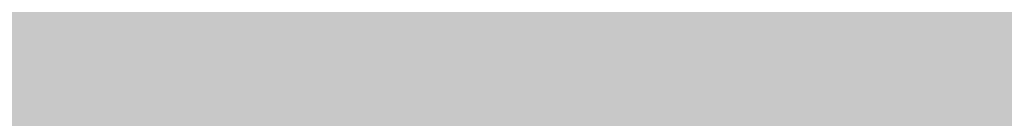
# Model space of a CAD drawing. Units: millimetres. Extents: x -22994 to 29398, y -19990 to 20176.
# Tile 87 of 135: x 229.428 to 230.597, y 83.328 to 83.446. Entities that reach past the tile are written whole.
import ezdxf
from ezdxf import colors
from ezdxf.entities.mleader import LeaderData, LeaderLine
from ezdxf.math import Vec2, Vec3

# ---------------------------------------------------------------- set-up
doc = ezdxf.new("R2010")
doc.units = ezdxf.units.MM
doc.header["$MEASUREMENT"] = 0
doc.layers.add('M-ANNO-TEXT', color=7, linetype='Continuous', lineweight=25)
doc.layers.add('M-DIMS', color=2, linetype='Continuous', lineweight=18)
doc.styles.get("Standard").update_dxf_attribs({"font": 'arial.ttf'})
doc.dimstyles.get("Standard").update_dxf_attribs({"dimtxt": 0.18, "dimasz": 10000, "dimexe": 0.18, "dimexo": 0.0625, "dimgap": 0.09, "dimtad": 0, "dimtih": 1, "dimtoh": 1, "dimdec": 0, "dimzin": 0, "dimdsep": 46, "dimtxsty": 'Standard', "dimcen": 0.09, "dimadec": 0, "dimazin": 0, "dimtfac": 1, "dimtdec": 0, "dimtofl": 0, "dimtmove": 0, "dimatfit": 3, "dimfxl": 1, "dimtolj": 1, "dimtzin": 0, "dimlwd": 30, "dimarcsym": 0})

# ---------------------------------------------------------------- blocks, each defined once
blk = doc.blocks.new('*D2')
at = {"layer": 'Defpoints', "color": 0, "transparency": 16777216}
for p in [(6.6773, 10.2713), (290.852, 10.2713), (290.852, -5.0787)]:
    blk.add_point(p, dxfattribs=at)
at = {"layer": 'M-DIMS', "color": 0, "lineweight": -2, "transparency": 16777216}
for p, q in [((6.6773, 10.2088), (6.6773, -5.2587)), ((290.852, 10.2088), (290.852, -5.2587))]:
    blk.add_line(p, q, dxfattribs=at)
at = {"layer": 'M-DIMS', "color": 0, "lineweight": 30, "transparency": 16777216}
for p, q in [((-9993.3227, -5.0787), (-19993.3227, -5.0787)), ((10290.852, -5.0787), (20290.852, -5.0787))]:
    blk.add_line(p, q, dxfattribs=at)
at = {"layer": 'M-DIMS', "color": 0, "transparency": 16777216}
for points in [[(-9993.3227, 1661.5879), (-9993.3227, -1671.7454), (6.6773, -5.0787)], [(10290.852, 1661.5879), (10290.852, -1671.7454), (290.852, -5.0787)]]:
    blk.add_solid(points, dxfattribs=at)
at = {"layer": 'M-DIMS', "color": 0, "transparency": 16777216, "insert": (148.7647, -5.0787), "char_height": 0.18, "attachment_point": 5}
blk.add_mtext('\\A1;284.2', dxfattribs=at)
blk = doc.blocks.new('*D3')
at = {"layer": 'Defpoints', "color": 0, "transparency": 16777216}
for p in [(110.2647, 204.1654), (110.2647, 176.3662), (95.8327, 127.967)]:
    blk.add_point(p, dxfattribs=at)
at = {"layer": 'M-DIMS', "color": 0, "lineweight": -2, "transparency": 16777216}
for p, q in [((95.8327, 128.0295), (95.8327, 204.3454)), ((110.2647, 176.4287), (110.2647, 204.3454))]:
    blk.add_line(p, q, dxfattribs=at)
at = {"layer": 'M-DIMS', "color": 0, "lineweight": 30, "transparency": 16777216}
for p, q in [((-9904.1673, 204.1654), (-19904.1673, 204.1654)), ((10110.2647, 204.1654), (20110.2647, 204.1654))]:
    blk.add_line(p, q, dxfattribs=at)
at = {"layer": 'M-DIMS', "color": 0, "transparency": 16777216}
for points in [[(-9904.1673, 1870.8321), (-9904.1673, -1462.5013), (95.8327, 204.1654)], [(10110.2647, 1870.8321), (10110.2647, -1462.5013), (110.2647, 204.1654)]]:
    blk.add_solid(points, dxfattribs=at)
at = {"layer": 'M-DIMS', "color": 0, "transparency": 16777216, "insert": (103.0487, 204.1654), "char_height": 0.18, "attachment_point": 5}
blk.add_mtext('\\A1;14.432', dxfattribs=at)
blk = doc.blocks.new('*D4')
at = {"layer": 'Defpoints', "color": 0, "transparency": 16777216}
for p in [(116.2647, 204.1654), (110.2647, 176.3662), (116.2647, 176.3662)]:
    blk.add_point(p, dxfattribs=at)
at = {"layer": 'M-DIMS', "color": 0, "lineweight": -2, "transparency": 16777216}
for p, q in [((110.2647, 176.4287), (110.2647, 204.3454)), ((116.2647, 176.4287), (116.2647, 204.3454))]:
    blk.add_line(p, q, dxfattribs=at)
at = {"layer": 'M-DIMS', "color": 0, "lineweight": 30, "transparency": 16777216}
for p, q in [((-9889.7353, 204.1654), (-19889.7353, 204.1654)), ((10116.2647, 204.1654), (20116.2647, 204.1654))]:
    blk.add_line(p, q, dxfattribs=at)
at = {"layer": 'M-DIMS', "color": 0, "transparency": 16777216}
for points in [[(-9889.7353, 1870.8321), (-9889.7353, -1462.5013), (110.2647, 204.1654)], [(10116.2647, 1870.8321), (10116.2647, -1462.5013), (116.2647, 204.1654)]]:
    blk.add_solid(points, dxfattribs=at)
at = {"layer": 'M-DIMS', "color": 0, "transparency": 16777216, "insert": (113.2647, 204.1654), "char_height": 0.18, "attachment_point": 5}
blk.add_mtext('\\A1;6', dxfattribs=at)
blk = doc.blocks.new('*D5')
at = {"layer": 'Defpoints', "color": 0, "transparency": 16777216}
for p in [(181.2647, 204.1654), (116.2647, 176.3662), (181.2647, 176.3662)]:
    blk.add_point(p, dxfattribs=at)
at = {"layer": 'M-DIMS', "color": 0, "lineweight": -2, "transparency": 16777216}
for p, q in [((116.2647, 176.4287), (116.2647, 204.3454)), ((181.2647, 176.4287), (181.2647, 204.3454))]:
    blk.add_line(p, q, dxfattribs=at)
at = {"layer": 'M-DIMS', "color": 0, "lineweight": 30, "transparency": 16777216}
for p, q in [((-9883.7353, 204.1654), (-19883.7353, 204.1654)), ((10181.2647, 204.1654), (20181.2647, 204.1654))]:
    blk.add_line(p, q, dxfattribs=at)
at = {"layer": 'M-DIMS', "color": 0, "transparency": 16777216}
for points in [[(-9883.7353, 1870.8321), (-9883.7353, -1462.5013), (116.2647, 204.1654)], [(10181.2647, 1870.8321), (10181.2647, -1462.5013), (181.2647, 204.1654)]]:
    blk.add_solid(points, dxfattribs=at)
at = {"layer": 'M-DIMS', "color": 0, "transparency": 16777216, "insert": (148.7647, 204.1654), "char_height": 0.18, "attachment_point": 5}
blk.add_mtext('\\A1;65', dxfattribs=at)
blk = doc.blocks.new('*D6')
at = {"layer": 'Defpoints', "color": 0, "transparency": 16777216}
for p in [(187.2647, 204.1654), (181.2647, 176.3662), (187.2647, 176.3662)]:
    blk.add_point(p, dxfattribs=at)
at = {"layer": 'M-DIMS', "color": 0, "lineweight": -2, "transparency": 16777216}
for p, q in [((181.2647, 176.4287), (181.2647, 204.3454)), ((187.2647, 176.4287), (187.2647, 204.3454))]:
    blk.add_line(p, q, dxfattribs=at)
at = {"layer": 'M-DIMS', "color": 0, "lineweight": 30, "transparency": 16777216}
for p, q in [((-9818.7353, 204.1654), (-19818.7353, 204.1654)), ((10187.2647, 204.1654), (20187.2647, 204.1654))]:
    blk.add_line(p, q, dxfattribs=at)
at = {"layer": 'M-DIMS', "color": 0, "transparency": 16777216}
for points in [[(-9818.7353, 1870.8321), (-9818.7353, -1462.5013), (181.2647, 204.1654)], [(10187.2647, 1870.8321), (10187.2647, -1462.5013), (187.2647, 204.1654)]]:
    blk.add_solid(points, dxfattribs=at)
at = {"layer": 'M-DIMS', "color": 0, "transparency": 16777216, "insert": (184.2647, 204.1654), "char_height": 0.18, "attachment_point": 5}
blk.add_mtext('\\A1;6', dxfattribs=at)
blk = doc.blocks.new('*D7')
at = {"layer": 'Defpoints', "color": 0, "transparency": 16777216}
for p in [(201.6967, 204.1654), (187.2647, 176.3662), (201.6967, 127.967)]:
    blk.add_point(p, dxfattribs=at)
at = {"layer": 'M-DIMS', "color": 0, "lineweight": -2, "transparency": 16777216}
for p, q in [((187.2647, 176.4287), (187.2647, 204.3454)), ((201.6967, 128.0295), (201.6967, 204.3454))]:
    blk.add_line(p, q, dxfattribs=at)
at = {"layer": 'M-DIMS', "color": 0, "lineweight": 30, "transparency": 16777216}
for p, q in [((-9812.7353, 204.1654), (-19812.7353, 204.1654)), ((10201.6967, 204.1654), (20201.6967, 204.1654))]:
    blk.add_line(p, q, dxfattribs=at)
at = {"layer": 'M-DIMS', "color": 0, "transparency": 16777216}
for points in [[(-9812.7353, 1870.8321), (-9812.7353, -1462.5013), (187.2647, 204.1654)], [(10201.6967, 1870.8321), (10201.6967, -1462.5013), (201.6967, 204.1654)]]:
    blk.add_solid(points, dxfattribs=at)
at = {"layer": 'M-DIMS', "color": 0, "transparency": 16777216, "insert": (194.4807, 204.1654), "char_height": 0.18, "attachment_point": 5}
blk.add_mtext('\\A1;14.432', dxfattribs=at)
blk = doc.blocks.new('*D8')
at = {"layer": 'Defpoints', "color": 0, "transparency": 16777216}
for p in [(227.6485, 204.1654), (227.6485, 146.7296), (201.6967, 127.967)]:
    blk.add_point(p, dxfattribs=at)
at = {"layer": 'M-DIMS', "color": 0, "lineweight": -2, "transparency": 16777216}
for p, q in [((201.6967, 128.0295), (201.6967, 204.3454)), ((227.6485, 146.7921), (227.6485, 204.3454))]:
    blk.add_line(p, q, dxfattribs=at)
at = {"layer": 'M-DIMS', "color": 0, "lineweight": 30, "transparency": 16777216}
for p, q in [((-9798.3033, 204.1654), (-19798.3033, 204.1654)), ((10227.6485, 204.1654), (20227.6485, 204.1654))]:
    blk.add_line(p, q, dxfattribs=at)
at = {"layer": 'M-DIMS', "color": 0, "transparency": 16777216}
for points in [[(-9798.3033, 1870.8321), (-9798.3033, -1462.5013), (201.6967, 204.1654)], [(10227.6485, 1870.8321), (10227.6485, -1462.5013), (227.6485, 204.1654)]]:
    blk.add_solid(points, dxfattribs=at)
at = {"layer": 'M-DIMS', "color": 0, "transparency": 16777216, "insert": (214.6726, 204.1654), "char_height": 0.18, "attachment_point": 5}
blk.add_mtext('\\A1;25.95', dxfattribs=at)
blk = doc.blocks.new('*D9')
at = {"layer": 'Defpoints', "color": 0, "transparency": 16777216}
for p in [(187.2647, 176.3662), (306.202, 176.3662), (290.852, 10.2713)]:
    blk.add_point(p, dxfattribs=at)
at = {"layer": 'M-DIMS', "color": 0, "lineweight": 30, "transparency": 16777216}
for p, q in [((306.202, 10176.3662), (306.202, 20176.3662)), ((306.202, -9989.7287), (306.202, -19989.7287))]:
    blk.add_line(p, q, dxfattribs=at)
at = {"layer": 'M-DIMS', "color": 0, "lineweight": -2, "transparency": 16777216}
for p, q in [((187.3272, 176.3662), (306.382, 176.3662)), ((290.9145, 10.2713), (306.382, 10.2713))]:
    blk.add_line(p, q, dxfattribs=at)
at = {"layer": 'M-DIMS', "color": 0, "transparency": 16777216}
for points in [[(-1360.4646, 10176.3662), (1972.8687, 10176.3662), (306.202, 176.3662)], [(-1360.4646, -9989.7287), (1972.8687, -9989.7287), (306.202, 10.2713)]]:
    blk.add_solid(points, dxfattribs=at)
at = {"layer": 'M-DIMS', "color": 0, "transparency": 16777216, "insert": (306.202, 93.3187), "char_height": 0.18, "attachment_point": 5}
blk.add_mtext('\\A1;166.1', dxfattribs=at)
blk = doc.blocks.new('*D10')
at = {"layer": 'Defpoints', "color": 0, "transparency": 16777216}
for p in [(125.6498, 136.0713), (133.3459, 136.0713), (133.3459, -5.0787)]:
    blk.add_point(p, dxfattribs=at)
at = {"layer": 'M-DIMS', "color": 0, "lineweight": -2, "transparency": 16777216}
for p, q in [((125.6498, 136.0088), (125.6498, -5.2587)), ((133.3459, 136.0088), (133.3459, -5.2587))]:
    blk.add_line(p, q, dxfattribs=at)
at = {"layer": 'M-DIMS', "color": 0, "lineweight": 30, "transparency": 16777216}
for p, q in [((-9874.3502, -5.0787), (-19874.3502, -5.0787)), ((10133.3459, -5.0787), (20133.3459, -5.0787))]:
    blk.add_line(p, q, dxfattribs=at)
at = {"layer": 'M-DIMS', "color": 0, "transparency": 16777216}
for points in [[(-9874.3502, 1661.5879), (-9874.3502, -1671.7454), (125.6498, -5.0787)], [(10133.3459, 1661.5879), (10133.3459, -1671.7454), (133.3459, -5.0787)]]:
    blk.add_solid(points, dxfattribs=at)
at = {"layer": 'M-DIMS', "color": 0, "transparency": 16777216, "insert": (129.4978, -5.0787), "char_height": 0.18, "attachment_point": 5}
blk.add_mtext('\\A1;7.696', dxfattribs=at)
blk = doc.blocks.new('*D11')
at = {"layer": 'Defpoints', "color": 0, "transparency": 16777216}
for p in [(133.3459, 136.0713), (135.6498, 136.0713), (135.6498, -5.0787)]:
    blk.add_point(p, dxfattribs=at)
at = {"layer": 'M-DIMS', "color": 0, "lineweight": -2, "transparency": 16777216}
for p, q in [((133.3459, 136.0088), (133.3459, -5.2587)), ((135.6498, 136.0088), (135.6498, -5.2587))]:
    blk.add_line(p, q, dxfattribs=at)
at = {"layer": 'M-DIMS', "color": 0, "lineweight": 30, "transparency": 16777216}
for p, q in [((-9866.6541, -5.0787), (-19866.6541, -5.0787)), ((10135.6498, -5.0787), (20135.6498, -5.0787))]:
    blk.add_line(p, q, dxfattribs=at)
at = {"layer": 'M-DIMS', "color": 0, "transparency": 16777216}
for points in [[(-9866.6541, 1661.5879), (-9866.6541, -1671.7454), (133.3459, -5.0787)], [(10135.6498, 1661.5879), (10135.6498, -1671.7454), (135.6498, -5.0787)]]:
    blk.add_solid(points, dxfattribs=at)
at = {"layer": 'M-DIMS', "color": 0, "transparency": 16777216, "insert": (134.4978, -5.0787), "char_height": 0.18, "attachment_point": 5}
blk.add_mtext('\\A1;2.304', dxfattribs=at)
blk = doc.blocks.new('*D12')
at = {"layer": 'Defpoints', "color": 0, "transparency": 16777216}
for p in [(135.6498, 136.0713), (145.6498, 136.0713), (145.6498, -5.0787)]:
    blk.add_point(p, dxfattribs=at)
at = {"layer": 'M-DIMS', "color": 0, "lineweight": -2, "transparency": 16777216}
for p, q in [((135.6498, 136.0088), (135.6498, -5.2587)), ((145.6498, 136.0088), (145.6498, -5.2587))]:
    blk.add_line(p, q, dxfattribs=at)
at = {"layer": 'M-DIMS', "color": 0, "lineweight": 30, "transparency": 16777216}
for p, q in [((-9864.3502, -5.0787), (-19864.3502, -5.0787)), ((10145.6498, -5.0787), (20145.6498, -5.0787))]:
    blk.add_line(p, q, dxfattribs=at)
at = {"layer": 'M-DIMS', "color": 0, "transparency": 16777216}
for points in [[(-9864.3502, 1661.5879), (-9864.3502, -1671.7454), (135.6498, -5.0787)], [(10145.6498, 1661.5879), (10145.6498, -1671.7454), (145.6498, -5.0787)]]:
    blk.add_solid(points, dxfattribs=at)
at = {"layer": 'M-DIMS', "color": 0, "transparency": 16777216, "insert": (140.6498, -5.0787), "char_height": 0.18, "attachment_point": 5}
blk.add_mtext('\\A1;10', dxfattribs=at)
blk = doc.blocks.new('*D13')
at = {"layer": 'Defpoints', "color": 0, "transparency": 16777216}
for p in [(145.6498, 136.0713), (155.6498, 136.0713), (155.6498, -5.0787)]:
    blk.add_point(p, dxfattribs=at)
at = {"layer": 'M-DIMS', "color": 0, "lineweight": -2, "transparency": 16777216}
for p, q in [((145.6498, 136.0088), (145.6498, -5.2587)), ((155.6498, 136.0088), (155.6498, -5.2587))]:
    blk.add_line(p, q, dxfattribs=at)
at = {"layer": 'M-DIMS', "color": 0, "lineweight": 30, "transparency": 16777216}
for p, q in [((-9854.3502, -5.0787), (-19854.3502, -5.0787)), ((10155.6498, -5.0787), (20155.6498, -5.0787))]:
    blk.add_line(p, q, dxfattribs=at)
at = {"layer": 'M-DIMS', "color": 0, "transparency": 16777216}
for points in [[(-9854.3502, 1661.5879), (-9854.3502, -1671.7454), (145.6498, -5.0787)], [(10155.6498, 1661.5879), (10155.6498, -1671.7454), (155.6498, -5.0787)]]:
    blk.add_solid(points, dxfattribs=at)
at = {"layer": 'M-DIMS', "color": 0, "transparency": 16777216, "insert": (150.6498, -5.0787), "char_height": 0.18, "attachment_point": 5}
blk.add_mtext('\\A1;10', dxfattribs=at)
blk = doc.blocks.new('*D14')
at = {"layer": 'Defpoints', "color": 0, "transparency": 16777216}
for p in [(155.6498, 136.0713), (165.6498, 136.0713), (165.6498, -5.0787)]:
    blk.add_point(p, dxfattribs=at)
at = {"layer": 'M-DIMS', "color": 0, "lineweight": -2, "transparency": 16777216}
for p, q in [((155.6498, 136.0088), (155.6498, -5.2587)), ((165.6498, 136.0088), (165.6498, -5.2587))]:
    blk.add_line(p, q, dxfattribs=at)
at = {"layer": 'M-DIMS', "color": 0, "lineweight": 30, "transparency": 16777216}
for p, q in [((-9844.3502, -5.0787), (-19844.3502, -5.0787)), ((10165.6498, -5.0787), (20165.6498, -5.0787))]:
    blk.add_line(p, q, dxfattribs=at)
at = {"layer": 'M-DIMS', "color": 0, "transparency": 16777216}
for points in [[(-9844.3502, 1661.5879), (-9844.3502, -1671.7454), (155.6498, -5.0787)], [(10165.6498, 1661.5879), (10165.6498, -1671.7454), (165.6498, -5.0787)]]:
    blk.add_solid(points, dxfattribs=at)
at = {"layer": 'M-DIMS', "color": 0, "transparency": 16777216, "insert": (160.6498, -5.0787), "char_height": 0.18, "attachment_point": 5}
blk.add_mtext('\\A1;10', dxfattribs=at)
blk = doc.blocks.new('*D15')
at = {"layer": 'Defpoints', "color": 0, "transparency": 16777216}
for p in [(173.3459, 154.788), (173.3459, 136.0713), (306.202, 136.0713)]:
    blk.add_point(p, dxfattribs=at)
at = {"layer": 'M-DIMS', "color": 0, "lineweight": 30, "transparency": 16777216}
for p, q in [((306.202, 10154.788), (306.202, 20154.788)), ((306.202, -9863.9287), (306.202, -19863.9287))]:
    blk.add_line(p, q, dxfattribs=at)
at = {"layer": 'M-DIMS', "color": 0, "lineweight": -2, "transparency": 16777216}
for p, q in [((173.4084, 154.788), (306.382, 154.788)), ((173.4084, 136.0713), (306.382, 136.0713))]:
    blk.add_line(p, q, dxfattribs=at)
at = {"layer": 'M-DIMS', "color": 0, "transparency": 16777216}
for points in [[(-1360.4646, 10154.788), (1972.8687, 10154.788), (306.202, 154.788)], [(-1360.4646, -9863.9287), (1972.8687, -9863.9287), (306.202, 136.0713)]]:
    blk.add_solid(points, dxfattribs=at)
at = {"layer": 'M-DIMS', "color": 0, "transparency": 16777216, "insert": (306.202, 145.4297), "char_height": 0.18, "attachment_point": 5}
blk.add_mtext('\\A1;18.717', dxfattribs=at)
blk = doc.blocks.new('*D16')
at = {"layer": 'Defpoints', "color": 0, "transparency": 16777216}
for p in [(120.1702, 204.1654), (110.4658, 48.0349), (120.1702, 48.0349)]:
    blk.add_point(p, dxfattribs=at)
at = {"layer": 'M-DIMS', "color": 0, "lineweight": -2, "transparency": 16777216}
for p, q in [((110.4658, 48.0974), (110.4658, 204.3454)), ((120.1702, 48.0974), (120.1702, 204.3454))]:
    blk.add_line(p, q, dxfattribs=at)
at = {"layer": 'M-DIMS', "color": 0, "lineweight": 30, "transparency": 16777216}
for p, q in [((-9889.5342, 204.1654), (-19889.5342, 204.1654)), ((10120.1702, 204.1654), (20120.1702, 204.1654))]:
    blk.add_line(p, q, dxfattribs=at)
at = {"layer": 'M-DIMS', "color": 0, "transparency": 16777216}
for points in [[(-9889.5342, 1870.8321), (-9889.5342, -1462.5013), (110.4658, 204.1654)], [(10120.1702, 1870.8321), (10120.1702, -1462.5013), (120.1702, 204.1654)]]:
    blk.add_solid(points, dxfattribs=at)
at = {"layer": 'M-DIMS', "color": 0, "transparency": 16777216, "insert": (115.318, 204.1654), "char_height": 0.18, "attachment_point": 5}
blk.add_mtext('\\A1;9.704', dxfattribs=at)
blk = doc.blocks.new('*D17')
at = {"layer": 'Defpoints', "color": 0, "transparency": 16777216}
for p in [(126.1702, 204.1654), (120.1702, 48.0349), (126.1702, 48.0349)]:
    blk.add_point(p, dxfattribs=at)
at = {"layer": 'M-DIMS', "color": 0, "lineweight": -2, "transparency": 16777216}
for p, q in [((120.1702, 48.0974), (120.1702, 204.3454)), ((126.1702, 48.0974), (126.1702, 204.3454))]:
    blk.add_line(p, q, dxfattribs=at)
at = {"layer": 'M-DIMS', "color": 0, "lineweight": 30, "transparency": 16777216}
for p, q in [((-9879.8298, 204.1654), (-19879.8298, 204.1654)), ((10126.1702, 204.1654), (20126.1702, 204.1654))]:
    blk.add_line(p, q, dxfattribs=at)
at = {"layer": 'M-DIMS', "color": 0, "transparency": 16777216}
for points in [[(-9879.8298, 1870.8321), (-9879.8298, -1462.5013), (120.1702, 204.1654)], [(10126.1702, 1870.8321), (10126.1702, -1462.5013), (126.1702, 204.1654)]]:
    blk.add_solid(points, dxfattribs=at)
at = {"layer": 'M-DIMS', "color": 0, "transparency": 16777216, "insert": (123.1702, 204.1654), "char_height": 0.18, "attachment_point": 5}
blk.add_mtext('\\A1;6', dxfattribs=at)
blk = doc.blocks.new('*D18')
at = {"layer": 'Defpoints', "color": 0, "transparency": 16777216}
for p in [(132.1702, 204.1654), (126.1702, 48.0349), (132.1702, 48.0349)]:
    blk.add_point(p, dxfattribs=at)
at = {"layer": 'M-DIMS', "color": 0, "lineweight": -2, "transparency": 16777216}
for p, q in [((126.1702, 48.0974), (126.1702, 204.3454)), ((132.1702, 48.0974), (132.1702, 204.3454))]:
    blk.add_line(p, q, dxfattribs=at)
at = {"layer": 'M-DIMS', "color": 0, "lineweight": 30, "transparency": 16777216}
for p, q in [((-9873.8298, 204.1654), (-19873.8298, 204.1654)), ((10132.1702, 204.1654), (20132.1702, 204.1654))]:
    blk.add_line(p, q, dxfattribs=at)
at = {"layer": 'M-DIMS', "color": 0, "transparency": 16777216}
for points in [[(-9873.8298, 1870.8321), (-9873.8298, -1462.5013), (126.1702, 204.1654)], [(10132.1702, 1870.8321), (10132.1702, -1462.5013), (132.1702, 204.1654)]]:
    blk.add_solid(points, dxfattribs=at)
at = {"layer": 'M-DIMS', "color": 0, "transparency": 16777216, "insert": (129.1702, 204.1654), "char_height": 0.18, "attachment_point": 5}
blk.add_mtext('\\A1;6', dxfattribs=at)
blk = doc.blocks.new('*D19')
at = {"layer": 'Defpoints', "color": 0, "transparency": 16777216}
for p in [(138.1702, 204.1654), (132.1702, 48.0349), (138.1702, 48.0349)]:
    blk.add_point(p, dxfattribs=at)
at = {"layer": 'M-DIMS', "color": 0, "lineweight": -2, "transparency": 16777216}
for p, q in [((132.1702, 48.0974), (132.1702, 204.3454)), ((138.1702, 48.0974), (138.1702, 204.3454))]:
    blk.add_line(p, q, dxfattribs=at)
at = {"layer": 'M-DIMS', "color": 0, "lineweight": 30, "transparency": 16777216}
for p, q in [((-9867.8298, 204.1654), (-19867.8298, 204.1654)), ((10138.1702, 204.1654), (20138.1702, 204.1654))]:
    blk.add_line(p, q, dxfattribs=at)
at = {"layer": 'M-DIMS', "color": 0, "transparency": 16777216}
for points in [[(-9867.8298, 1870.8321), (-9867.8298, -1462.5013), (132.1702, 204.1654)], [(10138.1702, 1870.8321), (10138.1702, -1462.5013), (138.1702, 204.1654)]]:
    blk.add_solid(points, dxfattribs=at)
at = {"layer": 'M-DIMS', "color": 0, "transparency": 16777216, "insert": (135.1702, 204.1654), "char_height": 0.18, "attachment_point": 5}
blk.add_mtext('\\A1;6', dxfattribs=at)
blk = doc.blocks.new('*D20')
at = {"layer": 'Defpoints', "color": 0, "transparency": 16777216}
for p in [(144.1702, 204.1654), (138.1702, 48.0349), (144.1702, 48.0349)]:
    blk.add_point(p, dxfattribs=at)
at = {"layer": 'M-DIMS', "color": 0, "lineweight": -2, "transparency": 16777216}
for p, q in [((138.1702, 48.0974), (138.1702, 204.3454)), ((144.1702, 48.0974), (144.1702, 204.3454))]:
    blk.add_line(p, q, dxfattribs=at)
at = {"layer": 'M-DIMS', "color": 0, "lineweight": 30, "transparency": 16777216}
for p, q in [((-9861.8298, 204.1654), (-19861.8298, 204.1654)), ((10144.1702, 204.1654), (20144.1702, 204.1654))]:
    blk.add_line(p, q, dxfattribs=at)
at = {"layer": 'M-DIMS', "color": 0, "transparency": 16777216}
for points in [[(-9861.8298, 1870.8321), (-9861.8298, -1462.5013), (138.1702, 204.1654)], [(10144.1702, 1870.8321), (10144.1702, -1462.5013), (144.1702, 204.1654)]]:
    blk.add_solid(points, dxfattribs=at)
at = {"layer": 'M-DIMS', "color": 0, "transparency": 16777216, "insert": (141.1702, 204.1654), "char_height": 0.18, "attachment_point": 5}
blk.add_mtext('\\A1;6', dxfattribs=at)
blk = doc.blocks.new('*D21')
at = {"layer": 'Defpoints', "color": 0, "transparency": 16777216}
for p in [(149.1157, 204.1654), (144.1702, 48.0349), (149.1157, 48.0349)]:
    blk.add_point(p, dxfattribs=at)
at = {"layer": 'M-DIMS', "color": 0, "lineweight": -2, "transparency": 16777216}
for p, q in [((144.1702, 48.0974), (144.1702, 204.3454)), ((149.1157, 48.0974), (149.1157, 204.3454))]:
    blk.add_line(p, q, dxfattribs=at)
at = {"layer": 'M-DIMS', "color": 0, "lineweight": 30, "transparency": 16777216}
for p, q in [((-9855.8298, 204.1654), (-19855.8298, 204.1654)), ((10149.1157, 204.1654), (20149.1157, 204.1654))]:
    blk.add_line(p, q, dxfattribs=at)
at = {"layer": 'M-DIMS', "color": 0, "transparency": 16777216}
for points in [[(-9855.8298, 1870.8321), (-9855.8298, -1462.5013), (144.1702, 204.1654)], [(10149.1157, 1870.8321), (10149.1157, -1462.5013), (149.1157, 204.1654)]]:
    blk.add_solid(points, dxfattribs=at)
at = {"layer": 'M-DIMS', "color": 0, "transparency": 16777216, "insert": (146.6429, 204.1654), "char_height": 0.18, "attachment_point": 5}
blk.add_mtext('\\A1;4.945', dxfattribs=at)
blk = doc.blocks.new('*D22')
at = {"layer": 'Defpoints', "color": 0, "transparency": 16777216}
for p in [(149.1157, 30.9895), (155.1157, 30.9895), (155.1157, -5.0787)]:
    blk.add_point(p, dxfattribs=at)
at = {"layer": 'M-DIMS', "color": 0, "lineweight": -2, "transparency": 16777216}
for p, q in [((149.1157, 30.927), (149.1157, -5.2587)), ((155.1157, 30.927), (155.1157, -5.2587))]:
    blk.add_line(p, q, dxfattribs=at)
at = {"layer": 'M-DIMS', "color": 0, "lineweight": 30, "transparency": 16777216}
for p, q in [((-9850.8843, -5.0787), (-19850.8843, -5.0787)), ((10155.1157, -5.0787), (20155.1157, -5.0787))]:
    blk.add_line(p, q, dxfattribs=at)
at = {"layer": 'M-DIMS', "color": 0, "transparency": 16777216}
for points in [[(-9850.8843, 1661.5879), (-9850.8843, -1671.7454), (149.1157, -5.0787)], [(10155.1157, 1661.5879), (10155.1157, -1671.7454), (155.1157, -5.0787)]]:
    blk.add_solid(points, dxfattribs=at)
at = {"layer": 'M-DIMS', "color": 0, "transparency": 16777216, "insert": (152.1157, -5.0787), "char_height": 0.18, "attachment_point": 5}
blk.add_mtext('\\A1;6', dxfattribs=at)
blk = doc.blocks.new('*D23')
at = {"layer": 'Defpoints', "color": 0, "transparency": 16777216}
for p in [(155.1157, 30.9895), (161.1157, 30.9895), (161.1157, -5.0787)]:
    blk.add_point(p, dxfattribs=at)
at = {"layer": 'M-DIMS', "color": 0, "lineweight": -2, "transparency": 16777216}
for p, q in [((155.1157, 30.927), (155.1157, -5.2587)), ((161.1157, 30.927), (161.1157, -5.2587))]:
    blk.add_line(p, q, dxfattribs=at)
at = {"layer": 'M-DIMS', "color": 0, "lineweight": 30, "transparency": 16777216}
for p, q in [((-9844.8843, -5.0787), (-19844.8843, -5.0787)), ((10161.1157, -5.0787), (20161.1157, -5.0787))]:
    blk.add_line(p, q, dxfattribs=at)
at = {"layer": 'M-DIMS', "color": 0, "transparency": 16777216}
for points in [[(-9844.8843, 1661.5879), (-9844.8843, -1671.7454), (155.1157, -5.0787)], [(10161.1157, 1661.5879), (10161.1157, -1671.7454), (161.1157, -5.0787)]]:
    blk.add_solid(points, dxfattribs=at)
at = {"layer": 'M-DIMS', "color": 0, "transparency": 16777216, "insert": (158.1157, -5.0787), "char_height": 0.18, "attachment_point": 5}
blk.add_mtext('\\A1;6', dxfattribs=at)
blk = doc.blocks.new('*D24')
at = {"layer": 'Defpoints', "color": 0, "transparency": 16777216}
for p in [(161.1157, 30.9895), (166.4387, 30.9895), (166.4387, -5.0787)]:
    blk.add_point(p, dxfattribs=at)
at = {"layer": 'M-DIMS', "color": 0, "lineweight": -2, "transparency": 16777216}
for p, q in [((161.1157, 30.927), (161.1157, -5.2587)), ((166.4387, 30.927), (166.4387, -5.2587))]:
    blk.add_line(p, q, dxfattribs=at)
at = {"layer": 'M-DIMS', "color": 0, "lineweight": 30, "transparency": 16777216}
for p, q in [((-9838.8843, -5.0787), (-19838.8843, -5.0787)), ((10166.4387, -5.0787), (20166.4387, -5.0787))]:
    blk.add_line(p, q, dxfattribs=at)
at = {"layer": 'M-DIMS', "color": 0, "transparency": 16777216}
for points in [[(-9838.8843, 1661.5879), (-9838.8843, -1671.7454), (161.1157, -5.0787)], [(10166.4387, 1661.5879), (10166.4387, -1671.7454), (166.4387, -5.0787)]]:
    blk.add_solid(points, dxfattribs=at)
at = {"layer": 'M-DIMS', "color": 0, "transparency": 16777216, "insert": (163.7772, -5.0787), "char_height": 0.18, "attachment_point": 5}
blk.add_mtext('\\A1;5.323', dxfattribs=at)
blk = doc.blocks.new('*D25')
at = {"layer": 'Defpoints', "color": 0, "transparency": 16777216}
for p in [(166.4387, 30.9895), (172.4387, 30.9895), (172.4387, -5.0787)]:
    blk.add_point(p, dxfattribs=at)
at = {"layer": 'M-DIMS', "color": 0, "lineweight": -2, "transparency": 16777216}
for p, q in [((166.4387, 30.927), (166.4387, -5.2587)), ((172.4387, 30.927), (172.4387, -5.2587))]:
    blk.add_line(p, q, dxfattribs=at)
at = {"layer": 'M-DIMS', "color": 0, "lineweight": 30, "transparency": 16777216}
for p, q in [((-9833.5613, -5.0787), (-19833.5613, -5.0787)), ((10172.4387, -5.0787), (20172.4387, -5.0787))]:
    blk.add_line(p, q, dxfattribs=at)
at = {"layer": 'M-DIMS', "color": 0, "transparency": 16777216}
for points in [[(-9833.5613, 1661.5879), (-9833.5613, -1671.7454), (166.4387, -5.0787)], [(10172.4387, 1661.5879), (10172.4387, -1671.7454), (172.4387, -5.0787)]]:
    blk.add_solid(points, dxfattribs=at)
at = {"layer": 'M-DIMS', "color": 0, "transparency": 16777216, "insert": (169.4387, -5.0787), "char_height": 0.18, "attachment_point": 5}
blk.add_mtext('\\A1;6', dxfattribs=at)
blk = doc.blocks.new('*D26')
at = {"layer": 'Defpoints', "color": 0, "transparency": 16777216}
for p in [(172.4387, 30.9895), (178.4387, 30.9895), (178.4387, -5.0787)]:
    blk.add_point(p, dxfattribs=at)
at = {"layer": 'M-DIMS', "color": 0, "lineweight": -2, "transparency": 16777216}
for p, q in [((172.4387, 30.927), (172.4387, -5.2587)), ((178.4387, 30.927), (178.4387, -5.2587))]:
    blk.add_line(p, q, dxfattribs=at)
at = {"layer": 'M-DIMS', "color": 0, "lineweight": 30, "transparency": 16777216}
for p, q in [((-9827.5613, -5.0787), (-19827.5613, -5.0787)), ((10178.4387, -5.0787), (20178.4387, -5.0787))]:
    blk.add_line(p, q, dxfattribs=at)
at = {"layer": 'M-DIMS', "color": 0, "transparency": 16777216}
for points in [[(-9827.5613, 1661.5879), (-9827.5613, -1671.7454), (172.4387, -5.0787)], [(10178.4387, 1661.5879), (10178.4387, -1671.7454), (178.4387, -5.0787)]]:
    blk.add_solid(points, dxfattribs=at)
at = {"layer": 'M-DIMS', "color": 0, "transparency": 16777216, "insert": (175.4387, -5.0787), "char_height": 0.18, "attachment_point": 5}
blk.add_mtext('\\A1;6', dxfattribs=at)
blk = doc.blocks.new('*D27')
at = {"layer": 'Defpoints', "color": 0, "transparency": 16777216}
for p in [(178.4387, 30.9895), (188.1175, 30.9895), (188.1175, -5.0787)]:
    blk.add_point(p, dxfattribs=at)
at = {"layer": 'M-DIMS', "color": 0, "lineweight": -2, "transparency": 16777216}
for p, q in [((178.4387, 30.927), (178.4387, -5.2587)), ((188.1175, 30.927), (188.1175, -5.2587))]:
    blk.add_line(p, q, dxfattribs=at)
at = {"layer": 'M-DIMS', "color": 0, "lineweight": 30, "transparency": 16777216}
for p, q in [((-9821.5613, -5.0787), (-19821.5613, -5.0787)), ((10188.1175, -5.0787), (20188.1175, -5.0787))]:
    blk.add_line(p, q, dxfattribs=at)
at = {"layer": 'M-DIMS', "color": 0, "transparency": 16777216}
for points in [[(-9821.5613, 1661.5879), (-9821.5613, -1671.7454), (178.4387, -5.0787)], [(10188.1175, 1661.5879), (10188.1175, -1671.7454), (188.1175, -5.0787)]]:
    blk.add_solid(points, dxfattribs=at)
at = {"layer": 'M-DIMS', "color": 0, "transparency": 16777216, "insert": (183.2781, -5.0787), "char_height": 0.18, "attachment_point": 5}
blk.add_mtext('\\A1;9.679', dxfattribs=at)
blk = doc.blocks.new('*D28')
at = {"layer": 'Defpoints', "color": 0, "transparency": 16777216}
for p in [(188.1175, 48.0349), (306.202, 48.0349), (188.1175, 30.9895)]:
    blk.add_point(p, dxfattribs=at)
at = {"layer": 'M-DIMS', "color": 0, "lineweight": 30, "transparency": 16777216}
for p, q in [((306.202, 10048.0349), (306.202, 20048.0349)), ((306.202, -9969.0105), (306.202, -19969.0105))]:
    blk.add_line(p, q, dxfattribs=at)
at = {"layer": 'M-DIMS', "color": 0, "lineweight": -2, "transparency": 16777216}
for p, q in [((188.18, 48.0349), (306.382, 48.0349)), ((188.18, 30.9895), (306.382, 30.9895))]:
    blk.add_line(p, q, dxfattribs=at)
at = {"layer": 'M-DIMS', "color": 0, "transparency": 16777216}
for points in [[(-1360.4646, 10048.0349), (1972.8687, 10048.0349), (306.202, 48.0349)], [(-1360.4646, -9969.0105), (1972.8687, -9969.0105), (306.202, 30.9895)]]:
    blk.add_solid(points, dxfattribs=at)
at = {"layer": 'M-DIMS', "color": 0, "transparency": 16777216, "insert": (306.202, 39.5122), "char_height": 0.18, "attachment_point": 5}
blk.add_mtext('\\A1;17.045', dxfattribs=at)
blk = doc.blocks.new('*D29')
at = {"layer": 'Defpoints', "color": 0, "transparency": 16777216}
for p in [(36.8006, 80.045), (64.0296, 80.045)]:
    blk.add_point(p, dxfattribs=at)
at = {"layer": 'M-DIMS', "color": 0, "lineweight": -2, "transparency": 16777216}
for p, q in [((50.4151, 79.955), (50.4151, 80.135)), ((50.3251, 80.045), (50.5051, 80.045))]:
    blk.add_line(p, q, dxfattribs=at)
at = {"layer": 'M-DIMS', "color": 0, "lineweight": 30, "transparency": 16777216}
blk.add_line((20064.0296, 80.0303), (10064.0296, 80.0377), dxfattribs=at)
at = {"layer": 'M-DIMS', "color": 0, "transparency": 16777216}
blk.add_solid([(10064.0309, 1746.7043), (10064.0284, -1586.629), (64.0296, 80.045)], dxfattribs=at)
at = {"layer": 'M-DIMS', "color": 0, "transparency": 16777216, "insert": (20064.5213, 80.0303), "char_height": 0.18, "attachment_point": 5}
blk.add_mtext('\\A1;∅27.23', dxfattribs=at)
blk = doc.blocks.new('*D30')
at = {"layer": 'Defpoints', "color": 0, "transparency": 16777216}
for p in [(216.3148, 146.7291), (238.9821, 146.73)]:
    blk.add_point(p, dxfattribs=at)
at = {"layer": 'M-DIMS', "color": 0, "lineweight": 30, "transparency": 16777216}
blk.add_line((20238.9821, 147.4959), (10238.9821, 147.1129), dxfattribs=at)
at = {"layer": 'M-DIMS', "color": 0, "lineweight": -2, "transparency": 16777216}
for p, q in [((227.6485, 146.6396), (227.6485, 146.8196)), ((227.5585, 146.7296), (227.7385, 146.7296))]:
    blk.add_line(p, q, dxfattribs=at)
at = {"layer": 'M-DIMS', "color": 0, "transparency": 16777216}
blk.add_solid([(10238.9183, 1813.7796), (10239.0459, -1519.5537), (238.9821, 146.73)], dxfattribs=at)
at = {"layer": 'M-DIMS', "color": 0, "transparency": 16777216, "insert": (20239.5436, 147.4959), "char_height": 0.18, "attachment_point": 5}
blk.add_mtext('\\A1;∅22.667', dxfattribs=at)
blk = doc.blocks.new('*D31')
at = {"layer": 'Defpoints', "color": 0, "transparency": 16777216}
for p in [(223.1641, 146.7291), (232.1328, 146.73)]:
    blk.add_point(p, dxfattribs=at)
at = {"layer": 'M-DIMS', "color": 0, "lineweight": 30, "transparency": 16777216}
blk.add_line((20232.1327, 148.6656), (10232.1328, 147.6978), dxfattribs=at)
at = {"layer": 'M-DIMS', "color": 0, "lineweight": -2, "transparency": 16777216}
for p, q in [((227.6485, 146.6396), (227.6485, 146.8196)), ((227.5585, 146.7296), (227.7385, 146.7296))]:
    blk.add_line(p, q, dxfattribs=at)
at = {"layer": 'M-DIMS', "color": 0, "transparency": 16777216}
blk.add_solid([(10231.9715, 1814.3645), (10232.2941, -1518.9688), (232.1328, 146.73)], dxfattribs=at)
at = {"layer": 'M-DIMS', "color": 0, "transparency": 16777216, "insert": (20232.6245, 148.6656), "char_height": 0.18, "attachment_point": 5}
blk.add_mtext('\\A1;∅8.969', dxfattribs=at)
blk = doc.blocks.new('*D33')
at = {"layer": 'Defpoints', "color": 0, "transparency": 16777216}
for p in [(229.5613, 154.3773), (232.9972, 153.3509)]:
    blk.add_point(p, dxfattribs=at)
at = {"layer": 'M-DIMS', "color": 0, "lineweight": -2, "transparency": 16777216}
for p, q in [((229.5613, 154.2873), (229.5613, 154.4673)), ((229.4713, 154.3773), (229.6513, 154.3773))]:
    blk.add_line(p, q, dxfattribs=at)
at = {"layer": 'M-DIMS', "color": 0, "lineweight": 30, "transparency": 16777216}
for p, q in [((19396.3388, -5570.8378), (9814.668, -2708.7434)), ((29396.3388, -5570.8378), (19396.3388, -5570.8378))]:
    blk.add_line(p, q, dxfattribs=at)
at = {"layer": 'M-DIMS', "color": 0, "transparency": 16777216}
blk.add_solid([(10291.6837, -1111.7983), (9337.6523, -4305.6886), (232.9972, 153.3509)], dxfattribs=at)
at = {"layer": 'M-DIMS', "color": 0, "transparency": 16777216, "insert": (29397.0125, -5570.8378), "char_height": 0.18, "attachment_point": 5}
blk.add_mtext('\\A1;6X R3.586', dxfattribs=at)
blk = doc.blocks.new('*D36')
at = {"layer": 'Defpoints', "color": 0, "transparency": 16777216}
for p in [(46.39, 31.3035), (46.3875, 26.5934)]:
    blk.add_point(p, dxfattribs=at)
at = {"layer": 'M-DIMS', "color": 0, "lineweight": 30, "transparency": 16777216}
for p, q in [((57.1499, 20031.3006), (51.77, 10031.302)), ((10057.1499, 20031.3006), (57.1499, 20031.3006))]:
    blk.add_line(p, q, dxfattribs=at)
at = {"layer": 'M-DIMS', "color": 0, "lineweight": -2, "transparency": 16777216}
for p, q in [((46.3887, 28.8585), (46.3887, 29.0385)), ((46.2987, 28.9485), (46.4787, 28.9485))]:
    blk.add_line(p, q, dxfattribs=at)
at = {"layer": 'M-DIMS', "color": 0, "transparency": 16777216}
blk.add_solid([(-1614.8965, 10032.1987), (1718.4364, 10030.4054), (46.39, 31.3035)], dxfattribs=at)
at = {"layer": 'M-DIMS', "color": 0, "transparency": 16777216, "insert": (10057.5542, 20031.3006), "char_height": 0.18, "attachment_point": 5}
blk.add_mtext('\\A1;∅4.71', dxfattribs=at)
blk = doc.blocks.new('*D37')
at = {"layer": 'Defpoints', "color": 0, "transparency": 16777216}
for p in [(54.8343, 118.6145), (59.4936, 118.614)]:
    blk.add_point(p, dxfattribs=at)
at = {"layer": 'M-DIMS', "color": 0, "lineweight": -2, "transparency": 16777216}
for p, q in [((57.1639, 118.5243), (57.1639, 118.7043)), ((57.0739, 118.6143), (57.2539, 118.6143))]:
    blk.add_line(p, q, dxfattribs=at)
at = {"layer": 'M-DIMS', "color": 0, "lineweight": 30, "transparency": 16777216}
blk.add_line((20059.4934, 116.2531), (10059.4935, 117.4336), dxfattribs=at)
at = {"layer": 'M-DIMS', "color": 0, "transparency": 16777216}
blk.add_solid([(10059.6902, 1784.1002), (10059.2968, -1549.2331), (59.4936, 118.614)], dxfattribs=at)
at = {"layer": 'M-DIMS', "color": 0, "transparency": 16777216, "insert": (20059.9852, 116.2531), "char_height": 0.18, "attachment_point": 5}
blk.add_mtext('\\A1;∅4.659', dxfattribs=at)

msp = doc.modelspace()

# ---------------------------------------------------------------- dimensions: what is measured, and where the dimension line sits
at = {"layer": 'M-DIMS'}
for base, p1, p2, override, picture, middle in [((306.202, 176.3662), (290.852, 10.2713), (187.2647, 176.3662), {"dimdec": 1, "dimlfac": 1, "dimrnd": 0, "dimzin": 0, "dimdsep": 46, "dimlunit": 2}, '*D9', (306.202, 93.3187)), ((306.202, 136.0713), (173.3459, 154.788), (173.3459, 136.0713), {"dimdec": 3, "dimlfac": 1, "dimrnd": 0, "dimzin": 0, "dimdsep": 46, "dimlunit": 2}, '*D15', (306.202, 145.4297)), ((306.202, 48.0349), (188.1175, 30.9895), (188.1175, 48.0349), {"dimdec": 3, "dimlfac": 1, "dimrnd": 0, "dimzin": 0, "dimdsep": 46, "dimlunit": 2}, '*D28', (306.202, 39.5122))]:
    dim = msp.add_linear_dim(base=base, p1=p1, p2=p2, angle=90, dimstyle='Standard', override=override, dxfattribs=at)
    dim.commit()
    dim.dimension.update_dxf_attribs({"geometry": picture, "text_midpoint": middle})
for p1, p2, override, picture, middle in [((46.3875, 26.5934), (46.39, 31.3035), {"dimdec": 2, "dimlfac": 1, "dimrnd": 0, "dimzin": 0, "dimdsep": 46, "dimlunit": 2}, '*D36', (10057.5542, 20031.3006)), ((223.1641, 146.7291), (232.1328, 146.73), {"dimdec": 3, "dimlfac": 1, "dimrnd": 0, "dimzin": 0, "dimdsep": 46, "dimlunit": 2}, '*D31', (20232.1327, 148.6656)), ((216.3148, 146.7291), (238.9821, 146.73), {"dimdec": 3, "dimlfac": 1, "dimrnd": 0, "dimzin": 0, "dimdsep": 46, "dimlunit": 2}, '*D30', (20238.9821, 147.4959))]:
    dim = msp.add_diameter_dim_2p(p1=p1, p2=p2, dimstyle='Standard', override=override, dxfattribs=at)
    dim.commit()
    dim.dimension.update_dxf_attribs({"geometry": picture, "text_midpoint": middle, "dimtype": 163})
for base, p1, p2, override, picture, middle in [((110.2647, 204.1654), (95.8327, 127.967), (110.2647, 176.3662), {"dimdec": 3, "dimlfac": 1, "dimrnd": 0, "dimzin": 0, "dimdsep": 46, "dimlunit": 2}, '*D3', (103.0487, 204.1654)), ((116.2647, 204.1654), (110.2647, 176.3662), (116.2647, 176.3662), {"dimdec": 0, "dimlfac": 1, "dimrnd": 0, "dimzin": 0, "dimdsep": 46, "dimlunit": 2}, '*D4', (113.2647, 204.1654)), ((120.1702, 204.1654), (110.4658, 48.0349), (120.1702, 48.0349), {"dimdec": 3, "dimlfac": 1, "dimrnd": 0, "dimzin": 0, "dimdsep": 46, "dimlunit": 2}, '*D16', (115.318, 204.1654)), ((181.2647, 204.1654), (116.2647, 176.3662), (181.2647, 176.3662), {"dimdec": 0, "dimlfac": 1, "dimrnd": 0, "dimzin": 0, "dimdsep": 46, "dimlunit": 2}, '*D5', (148.7647, 204.1654)), ((126.1702, 204.1654), (120.1702, 48.0349), (126.1702, 48.0349), {"dimdec": 0, "dimlfac": 1, "dimrnd": 0, "dimzin": 0, "dimdsep": 46, "dimlunit": 2}, '*D17', (123.1702, 204.1654)), ((132.1702, 204.1654), (126.1702, 48.0349), (132.1702, 48.0349), {"dimdec": 0, "dimlfac": 1, "dimrnd": 0, "dimzin": 0, "dimdsep": 46, "dimlunit": 2}, '*D18', (129.1702, 204.1654)), ((138.1702, 204.1654), (132.1702, 48.0349), (138.1702, 48.0349), {"dimdec": 0, "dimlfac": 1, "dimrnd": 0, "dimzin": 0, "dimdsep": 46, "dimlunit": 2}, '*D19', (135.1702, 204.1654)), ((144.1702, 204.1654), (138.1702, 48.0349), (144.1702, 48.0349), {"dimdec": 0, "dimlfac": 1, "dimrnd": 0, "dimzin": 0, "dimdsep": 46, "dimlunit": 2}, '*D20', (141.1702, 204.1654)), ((149.11567, 204.16539), (144.17023, 48.03494), (149.11567, 48.03494), {"dimdec": 3, "dimlfac": 1, "dimrnd": 0, "dimzin": 0, "dimdsep": 46, "dimlunit": 2}, '*D21', (146.64295, 204.16539)), ((187.2647, 204.1654), (181.2647, 176.3662), (187.2647, 176.3662), {"dimdec": 0, "dimlfac": 1, "dimrnd": 0, "dimzin": 0, "dimdsep": 46, "dimlunit": 2}, '*D6', (184.2647, 204.1654)), ((201.6967, 204.1654), (187.2647, 176.3662), (201.6967, 127.967), {"dimdec": 3, "dimlfac": 1, "dimrnd": 0, "dimzin": 0, "dimdsep": 46, "dimlunit": 2}, '*D7', (194.4807, 204.1654)), ((227.6485, 204.1654), (201.6967, 127.967), (227.6485, 146.7296), {"dimdec": 2, "dimlfac": 1, "dimrnd": 0, "dimzin": 0, "dimdsep": 46, "dimlunit": 2}, '*D8', (214.6726, 204.1654)), ((290.852, -5.0787), (6.6773, 10.2713), (290.852, 10.2713), {"dimdec": 1, "dimlfac": 1, "dimrnd": 0, "dimzin": 0, "dimdsep": 46, "dimlunit": 2}, '*D2', (148.7647, -5.0787)), ((133.3459, -5.0787), (125.6498, 136.0713), (133.3459, 136.0713), {"dimdec": 3, "dimlfac": 1, "dimrnd": 0, "dimzin": 0, "dimdsep": 46, "dimlunit": 2}, '*D10', (129.4978, -5.0787)), ((135.6498, -5.0787), (133.3459, 136.0713), (135.6498, 136.0713), {"dimdec": 3, "dimlfac": 1, "dimrnd": 0, "dimzin": 0, "dimdsep": 46, "dimlunit": 2}, '*D11', (134.4978, -5.0787)), ((145.6498, -5.0787), (135.6498, 136.0713), (145.6498, 136.0713), {"dimdec": 0, "dimlfac": 1, "dimrnd": 0, "dimzin": 0, "dimdsep": 46, "dimlunit": 2}, '*D12', (140.6498, -5.0787)), ((155.6498, -5.0787), (145.6498, 136.0713), (155.6498, 136.0713), {"dimdec": 0, "dimlfac": 1, "dimrnd": 0, "dimzin": 0, "dimdsep": 46, "dimlunit": 2}, '*D13', (150.6498, -5.0787)), ((155.1157, -5.0787), (149.1157, 30.9895), (155.1157, 30.9895), {"dimdec": 0, "dimlfac": 1, "dimrnd": 0, "dimzin": 0, "dimdsep": 46, "dimlunit": 2}, '*D22', (152.1157, -5.0787)), ((161.1157, -5.0787), (155.1157, 30.9895), (161.1157, 30.9895), {"dimdec": 0, "dimlfac": 1, "dimrnd": 0, "dimzin": 0, "dimdsep": 46, "dimlunit": 2}, '*D23', (158.1157, -5.0787)), ((165.6498, -5.0787), (155.6498, 136.0713), (165.6498, 136.0713), {"dimdec": 0, "dimlfac": 1, "dimrnd": 0, "dimzin": 0, "dimdsep": 46, "dimlunit": 2}, '*D14', (160.6498, -5.0787)), ((166.4387, -5.0787), (161.1157, 30.9895), (166.4387, 30.9895), {"dimdec": 3, "dimlfac": 1, "dimrnd": 0, "dimzin": 0, "dimdsep": 46, "dimlunit": 2}, '*D24', (163.7772, -5.0787)), ((172.4387, -5.0787), (166.4387, 30.9895), (172.4387, 30.9895), {"dimdec": 0, "dimlfac": 1, "dimrnd": 0, "dimzin": 0, "dimdsep": 46, "dimlunit": 2}, '*D25', (169.4387, -5.0787)), ((178.4387, -5.0787), (172.4387, 30.9895), (178.4387, 30.9895), {"dimdec": 0, "dimlfac": 1, "dimrnd": 0, "dimzin": 0, "dimdsep": 46, "dimlunit": 2}, '*D26', (175.4387, -5.0787)), ((188.1175, -5.0787), (178.4387, 30.9895), (188.1175, 30.9895), {"dimdec": 3, "dimlfac": 1, "dimrnd": 0, "dimzin": 0, "dimdsep": 46, "dimlunit": 2}, '*D27', (183.2781, -5.0787))]:
    dim = msp.add_linear_dim(base=base, p1=p1, p2=p2, dimstyle='Standard', override=override, dxfattribs=at)
    dim.commit()
    dim.dimension.update_dxf_attribs({"geometry": picture, "text_midpoint": middle})
for p1, p2, override, picture, middle in [((54.8343, 118.6145), (59.4936, 118.614), {"dimdec": 3, "dimlfac": 1, "dimrnd": 0, "dimzin": 0, "dimdsep": 46, "dimlunit": 2}, '*D37', (20059.4934, 116.2531)), ((36.8006, 80.045), (64.0296, 80.045), {"dimdec": 2, "dimlfac": 1, "dimrnd": 0, "dimzin": 0, "dimdsep": 46, "dimlunit": 2}, '*D29', (20064.0296, 80.0303))]:
    dim = msp.add_diameter_dim_2p(p1=p1, p2=p2, dimstyle='Standard', override=override, dxfattribs=at)
    dim.commit()
    dim.dimension.update_dxf_attribs({"geometry": picture, "text_midpoint": middle})
dim = msp.add_radius_dim(center=(229.5613, 154.3773), mpoint=(232.9972, 153.3509), text='6X <>', dimstyle='Standard', override={"dimdec": 3, "dimlfac": 1, "dimrnd": 0, "dimzin": 0, "dimdsep": 46, "dimlunit": 2}, dxfattribs=at)
dim.commit()
dim.dimension.update_dxf_attribs({"geometry": '*D33', "text_midpoint": (29397.0125, -5570.8378)})

# ---------------------------------------------------------------- leaders
at = {"layer": 'M-ANNO-TEXT'}
ml = msp.add_multileader_mtext('Standard', dxfattribs=at)
ml.set_content('combustion chamber', color=256)
ml.set_leader_properties()
ml.build(insert=Vec2(0, 0))
ml.multileader.update_dxf_attribs({"dogleg_length": 0.36, "arrow_head_size": 200})
ctx = ml.context
ctx.base_point, ctx.char_height, ctx.arrow_head_size, ctx.landing_gap_size, ctx.plane_origin = Vec3(215.7321, 57.9149), 3, 200, 0.09, Vec3(189.1175, 57.9149)
notes = []
notes.append((ctx, [(0, (1, 1, 0), (215.3721, 57.9149), (1, 0), 0.36, [(0, [(189.1175, 57.9149)], 0, [])])]))
ctx.mtext.insert, ctx.mtext.flow_direction = Vec3(215.8221, 59.4394), 5
for ctx, leaders in notes:
    for number, flags, end, landing, length, lines in leaders:
        leader = LeaderData()
        leader.index, (leader.has_last_leader_line, leader.has_dogleg_vector, leader.attachment_direction) = number, flags
        leader.last_leader_point, leader.dogleg_vector, leader.dogleg_length = Vec3(end), Vec3(landing), length
        for number, points, colour, breaks in lines:
            line = LeaderLine()
            line.index, line.vertices, line.color, line.breaks = number, Vec3.list(points), colors.encode_raw_color(colour), breaks
            leader.lines.append(line)
        ctx.leaders.append(leader)

doc.saveas('drawing.dxf')
